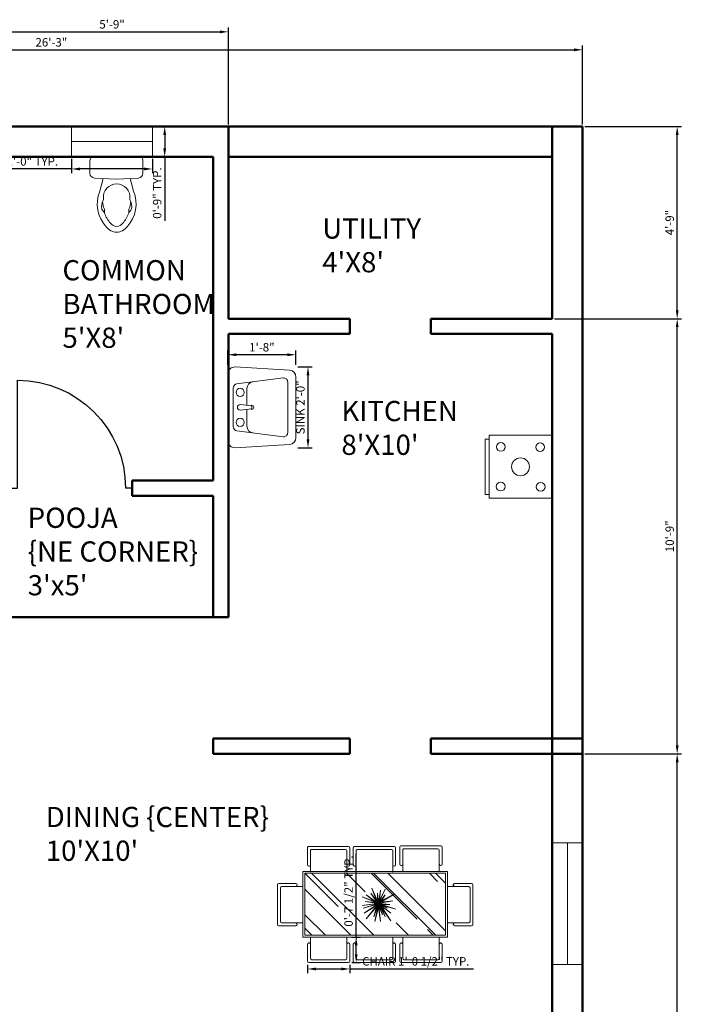
# Model space of a CAD drawing. Units: inches. Extents: x 20697 to 21575, y 6189 to 6822.
# Tile 4 of 7: x 20866 to 21063, y 6490 to 6782. Entities that reach past the tile are written whole.
import ezdxf

# ---------------------------------------------------------------- set-up
doc = ezdxf.new("R2010")
doc.units = ezdxf.units.IN
for name, color, linetype, lineweight in [('A-ANNO-DIMS', 2, 'Continuous', 18), ('A-AREA-IDEN', 7, 'Continuous', 18), ('A-DOOR', 4, 'Continuous', 25), ('A-EQPM', 9, 'Continuous', 18), ('A-FLOR-FIXT', 9, 'Continuous', 18), ('A-FURN', 8, 'Continuous', 18), ('A-GLAZ', 4, 'Continuous', 18), ('A-WALL', 7, 'Continuous', 50)]:
    doc.layers.add(name, color=color, linetype=linetype, lineweight=lineweight)
doc.styles.get("Standard").update_dxf_attribs({"font": 'arial.ttf'})
doc.dimstyles.new('ISO-25', dxfattribs={"dimtxt": 2.5, "dimasz": 2.5, "dimexe": 1.25, "dimexo": 0.625, "dimtad": 1, "dimdec": 0, "dimlunit": 3, "dimtxsty": 'Standard', "dimcen": 2.5, "dimadec": 0, "dimazin": 0, "dimtfac": 1, "dimtdec": 0, "dimtmove": 0, "dimatfit": 3, "dimfxl": 1, "dimarcsym": 0})

# ---------------------------------------------------------------- blocks, each defined once
blk = doc.blocks.new('*D5')
at = {"layer": 'A-ANNO-DIMS', "color": 0, "lineweight": -2, "transparency": 16777216}
for p, q in [((20718.29, 6750.68), (20718.29, 6774.03)), ((20720.79, 6772.78), (21030.79, 6772.78)), ((21033.29, 6750.68), (21033.29, 6774.03))]:
    blk.add_line(p, q, dxfattribs=at)
at = {"layer": 'A-ANNO-DIMS', "color": 0, "transparency": 16777216}
for points in [[(20720.79, 6773.19), (20720.79, 6772.36), (20718.29, 6772.78)], [(21030.79, 6773.19), (21030.79, 6772.36), (21033.29, 6772.78)]]:
    blk.add_solid(points, dxfattribs=at)
at = {"layer": 'Defpoints', "color": 0, "transparency": 16777216}
for p in [(21033.29, 6772.78), (20718.29, 6750.06), (21033.29, 6750.06)]:
    blk.add_point(p, dxfattribs=at)
at = {"layer": 'A-ANNO-DIMS', "color": 0, "transparency": 16777216, "insert": (20875.79, 6774.68), "char_height": 2.5, "attachment_point": 5}
blk.add_mtext('26\'-3"', dxfattribs=at)
blk = doc.blocks.new('A$C1308471B')
at = {"ltscale": 20}
for p, q in [((0, 0.4607), (0, 0.0186)), ((0.0354, 0.4793), (0.1495, 0.4793)), ((0.2013, 0.2397), (0.1923, 0.4384)), ((0.1957, 0.3639), (0.3109, 0.3953)), ((0.4982, 0.3575), (0.4822, 0.3709)), ((0.5021, 0.3528), (0.4724, 0.3528)), ((0.2013, 0.2397), (0.1923, 0.0409)), ((0.1959, 0.1193), (0.3109, 0.0879)), ((0.5021, 0.1304), (0.4724, 0.1304)), ((0.4982, 0.1257), (0.4822, 0.1123)), ((0.0354, 0), (0.1495, 0))]:
    blk.add_line(p, q, dxfattribs=at)
for centre, radius, start, end in [((0.006, 0.4607), 0.006, 136.52689, 180), ((0.0354, 0.4328), 0.0465, 90, 136.52689), ((0.1495, 0.4365), 0.0429, 2.57554, 90), ((0.3654, 0.2416), 0.1206, 83.35226, 180), ((0.4248, 0.1104), 0.3068, 47.41345, 111.79241), ((0.3823, 0.3868), 0.0255, 263.35226, 298.57415), ((0.4494, 0.2636), 0.1148, 79.39683, 118.57415), ((0.405, 0.2159), 0.153, 63.50202, 90.45216), ((0.4658, 0.3513), 0.0255, 50, 79.39683), ((0.5146, 0.377), 0.0255, 230, 251.38812), ((0.5021, 0.3273), 0.0255, 70.3751, 90), ((0.4248, 0.1104), 0.2558, 46.61198, 70.3751), ((0.5654, 0.2416), 0.065, 0, 57.29738), ((0.5654, 0.2416), 0.116, 0, 54.71147), ((0.3654, 0.2416), 0.1206, 180, 276.64774), ((0.4248, 0.3728), 0.2558, 289.6249, 313.38802), ((0.5654, 0.2416), 0.065, 302.70262, 0), ((0.5654, 0.2416), 0.116, 305.28853, 0), ((0.4248, 0.3728), 0.3068, 248.20759, 312.58655), ((0.3823, 0.0964), 0.0255, 61.42585, 96.64774), ((0.4494, 0.2196), 0.1148, 241.42585, 280.60317), ((0.405, 0.2673), 0.153, 269.54784, 296.49798), ((0.4658, 0.1319), 0.0255, 280.60317, 310), ((0.5146, 0.1062), 0.0255, 108.61188, 130), ((0.5021, 0.1559), 0.0255, 270, 289.6249), ((0.006, 0.0186), 0.006, 180, 223.47311), ((0.0354, 0.0465), 0.0465, 223.47311, 270), ((0.1495, 0.0429), 0.0429, 270, 357.42446)]:
    blk.add_arc(centre, radius, start, end, dxfattribs=at)
blk = doc.blocks.new('A$C2BB73538')
for p, q in [((0, 0.3474), (0.0187, 0.0365)), ((0.0388, 0.3886), (0.4225, 0.3886)), ((0.1191, 0.3575), (0.3422, 0.3575)), ((0.4613, 0.3474), (0.4427, 0.0365)), ((0.096, 0.3371), (0.063, 0.0728)), ((0.2151, 0.3186), (0.2229, 0.2526)), ((0.2384, 0.2526), (0.2462, 0.3186)), ((0.3653, 0.3371), (0.3984, 0.0728)), ((0.1231, 0.2798), (0.2197, 0.2798)), ((0.2229, 0.2526), (0.2384, 0.2526)), ((0.2416, 0.2798), (0.3382, 0.2798)), ((0.3752, 0.0466), (0.0861, 0.0466)), ((0.4039, 0), (0.0574, 0))]:
    blk.add_line(p, q)
for centre in [(0.1452, 0.3186), (0.3161, 0.3186)]:
    blk.add_circle(centre, 0.0233)
for centre, radius, start, end in [((0.0388, 0.3497), 0.0389, 90, 183.4336), ((0.1191, 0.3342), 0.0233, 90, 172.875), ((0.3422, 0.3342), 0.0233, 7.125, 90), ((0.3422, 0.3342), 0.0233, 7.125, 90), ((0.4225, 0.3497), 0.0389, 356.5664, 90), ((0.2307, 0.3186), 0.0155, 0, 180), ((0.1231, 0.2409), 0.0389, 90, 172.875), ((0.2307, 0.2526), 0.0117, 138.1701, 41.8299), ((0.3382, 0.2409), 0.0389, 7.125, 90), ((0.0861, 0.0699), 0.0233, 172.875, 270), ((0.3752, 0.0699), 0.0233, 270, 7.125), ((0.0574, 0.0389), 0.0389, 183.4336, 270), ((0.4039, 0.0389), 0.0389, 270, 356.5664)]:
    blk.add_arc(centre, radius, start, end)
blk = doc.blocks.new('DOOR-SWING-36')
for p, q in [((34, 0), (34, 32)), ((0, 0), (2, 0)), ((36, 0), (34, 0))]:
    blk.add_line(p, q)
blk.add_arc((34, 0), 32, 90, 180)
blk = doc.blocks.new('WIN-36X9')
for p, q in [((0, 9), (36, 9)), ((0, 0), (0, 9)), ((36, 9), (36, 0)), ((0, 4.5), (36, 4.5)), ((36, 0), (0, 0))]:
    blk.add_line(p, q)
blk = doc.blocks.new('WIN-24X9')
for p, q in [((0, 9), (24, 9)), ((0, 0), (0, 9)), ((24, 9), (24, 0)), ((0, 4.5), (24, 4.5)), ((24, 0), (0, 0))]:
    blk.add_line(p, q)
blk = doc.blocks.new('CHAIR-DINING')
for p, q in [((0.87, 1.26), (0.87, 7.58)), ((11.69, 7.58), (11.69, 1.26)), ((0, 0.39), (0, 5.43)), ((0.48, 5.82), (0.39, 5.82)), ((12.17, 5.82), (12.08, 5.82)), ((12.56, 5.43), (12.56, 0.39)), ((11.3, 0.87), (1.26, 0.87)), ((12.17, 0), (0.39, 0))]:
    blk.add_line(p, q)
for centre, start, end in [((0.39, 5.43), 90, 180), ((0.48, 5.43), 0, 90), ((12.08, 5.43), 90, 180), ((12.17, 5.43), 0, 90), ((0.39, 0.39), 180, 270), ((1.26, 1.26), 180, 270), ((11.3, 1.26), 270, 0), ((12.17, 0.39), 270, 0)]:
    blk.add_arc(centre, 0.39, start, end)
blk = doc.blocks.new('*D22')
at = {"layer": 'A-ANNO-DIMS', "color": 0, "lineweight": -2, "transparency": 16777216}
for p, q in [((20951.72, 6501.55), (20951.72, 6499.04)), ((20964.28, 6501.55), (20964.28, 6499.04)), ((20954.22, 6500.29), (20961.78, 6500.29)), ((20964.28, 6500.29), (21000.9, 6500.29))]:
    blk.add_line(p, q, dxfattribs=at)
at = {"layer": 'A-ANNO-DIMS', "color": 0, "transparency": 16777216}
for points in [[(20954.22, 6500.7), (20954.22, 6499.87), (20951.72, 6500.29)], [(20961.78, 6500.7), (20961.78, 6499.87), (20964.28, 6500.29)]]:
    blk.add_solid(points, dxfattribs=at)
at = {"layer": 'Defpoints', "color": 0, "transparency": 16777216}
for p in [(20951.72, 6502.17), (20964.28, 6502.17), (20964.28, 6500.29)]:
    blk.add_point(p, dxfattribs=at)
at = {"layer": 'A-ANNO-DIMS', "color": 0, "transparency": 16777216, "insert": (20983.84, 6502.21), "char_height": 2.5, "attachment_point": 5}
blk.add_mtext('CHAIR 1\'-0 1/2" TYP.', dxfattribs=at)
blk = doc.blocks.new('*D23')
at = {"layer": 'A-ANNO-DIMS', "color": 0, "lineweight": -2, "transparency": 16777216}
for p, q in [((20966.16, 6509.75), (20966.16, 6534.56)), ((20964.9, 6509.75), (20967.41, 6509.75)), ((20966.16, 6504.67), (20966.16, 6507.25)), ((20964.9, 6502.17), (20967.41, 6502.17))]:
    blk.add_line(p, q, dxfattribs=at)
at = {"layer": 'A-ANNO-DIMS', "color": 0, "transparency": 16777216}
for points in [[(20965.74, 6507.25), (20966.58, 6507.25), (20966.16, 6509.75)], [(20965.74, 6504.67), (20966.58, 6504.67), (20966.16, 6502.17)]]:
    blk.add_solid(points, dxfattribs=at)
at = {"layer": 'Defpoints', "color": 0, "transparency": 16777216}
for p in [(20964.28, 6509.75), (20966.16, 6509.75), (20964.28, 6502.17)]:
    blk.add_point(p, dxfattribs=at)
at = {"layer": 'A-ANNO-DIMS', "color": 0, "transparency": 16777216, "insert": (20964.24, 6523.4), "char_height": 2.5, "attachment_point": 5, "rotation": 90}
blk.add_mtext('0\'-7 1/2" TYP.', dxfattribs=at)
blk = doc.blocks.new('*D28')
at = {"layer": 'A-ANNO-DIMS', "color": 0, "lineweight": -2, "transparency": 16777216}
for p, q in [((20881.79, 6740.43), (20881.79, 6736.21)), ((20905.79, 6740.43), (20905.79, 6736.21)), ((20881.79, 6737.46), (20836.34, 6737.46)), ((20903.29, 6737.46), (20884.29, 6737.46))]:
    blk.add_line(p, q, dxfattribs=at)
at = {"layer": 'A-ANNO-DIMS', "color": 0, "transparency": 16777216}
for points in [[(20884.29, 6737.87), (20884.29, 6737.04), (20881.79, 6737.46)], [(20903.29, 6737.87), (20903.29, 6737.04), (20905.79, 6737.46)]]:
    blk.add_solid(points, dxfattribs=at)
at = {"layer": 'Defpoints', "color": 0, "transparency": 16777216}
for p in [(20881.79, 6741.06), (20905.79, 6741.06), (20881.79, 6737.46)]:
    blk.add_point(p, dxfattribs=at)
at = {"layer": 'A-ANNO-DIMS', "color": 0, "transparency": 16777216, "insert": (20857.81, 6739.37), "char_height": 2.5, "attachment_point": 5}
blk.add_mtext('BATH WINDOW 2\'-0" TYP.', dxfattribs=at)
blk = doc.blocks.new('*D29')
at = {"layer": 'A-ANNO-DIMS', "color": 0, "lineweight": -2, "transparency": 16777216}
for p, q in [((20906.42, 6750.06), (20910.64, 6750.06)), ((20909.39, 6747.56), (20909.39, 6743.56)), ((20906.42, 6741.06), (20910.64, 6741.06)), ((20909.39, 6741.06), (20909.39, 6722.07))]:
    blk.add_line(p, q, dxfattribs=at)
at = {"layer": 'A-ANNO-DIMS', "color": 0, "transparency": 16777216}
for points in [[(20908.98, 6747.56), (20909.81, 6747.56), (20909.39, 6750.06)], [(20908.98, 6743.56), (20909.81, 6743.56), (20909.39, 6741.06)]]:
    blk.add_solid(points, dxfattribs=at)
at = {"layer": 'Defpoints', "color": 0, "transparency": 16777216}
for p in [(20905.79, 6750.06), (20905.79, 6741.06), (20909.39, 6741.06)]:
    blk.add_point(p, dxfattribs=at)
at = {"layer": 'A-ANNO-DIMS', "color": 0, "transparency": 16777216, "insert": (20907.49, 6730.31), "char_height": 2.5, "attachment_point": 5, "rotation": 90}
blk.add_mtext('0\'-9" TYP.', dxfattribs=at)
blk = doc.blocks.new('*D50')
at = {"layer": 'A-ANNO-DIMS', "color": 0, "lineweight": -2, "transparency": 16777216}
for p, q in [((20948.91, 6678.78), (20953.14, 6678.78)), ((20951.89, 6657.28), (20951.89, 6676.28)), ((20948.91, 6654.78), (20953.14, 6654.78))]:
    blk.add_line(p, q, dxfattribs=at)
at = {"layer": 'A-ANNO-DIMS', "color": 0, "transparency": 16777216}
for points in [[(20951.47, 6676.28), (20952.3, 6676.28), (20951.89, 6678.78)], [(20951.47, 6657.28), (20952.3, 6657.28), (20951.89, 6654.78)]]:
    blk.add_solid(points, dxfattribs=at)
at = {"layer": 'Defpoints', "color": 0, "transparency": 16777216}
for p in [(20948.29, 6678.78), (20951.89, 6678.78), (20948.29, 6654.78)]:
    blk.add_point(p, dxfattribs=at)
at = {"layer": 'A-ANNO-DIMS', "color": 0, "transparency": 16777216, "insert": (20949.97, 6666.78), "char_height": 2.5, "attachment_point": 5, "rotation": 90}
blk.add_mtext('SINK 2\'-0"', dxfattribs=at)
blk = doc.blocks.new('*D51')
at = {"layer": 'A-ANNO-DIMS', "color": 0, "lineweight": -2, "transparency": 16777216}
for p, q in [((20928.13, 6679.41), (20928.13, 6683.63)), ((20945.79, 6682.38), (20930.63, 6682.38)), ((20948.29, 6679.41), (20948.29, 6683.63))]:
    blk.add_line(p, q, dxfattribs=at)
at = {"layer": 'A-ANNO-DIMS', "color": 0, "transparency": 16777216}
for points in [[(20930.63, 6682.8), (20930.63, 6681.97), (20928.13, 6682.38)], [(20945.79, 6682.8), (20945.79, 6681.97), (20948.29, 6682.38)]]:
    blk.add_solid(points, dxfattribs=at)
at = {"layer": 'Defpoints', "color": 0, "transparency": 16777216}
for p in [(20928.13, 6682.38), (20928.13, 6678.78), (20948.29, 6678.78)]:
    blk.add_point(p, dxfattribs=at)
at = {"layer": 'A-ANNO-DIMS', "color": 0, "transparency": 16777216, "insert": (20938.21, 6684.28), "char_height": 2.5, "attachment_point": 5}
blk.add_mtext('1\'-8"', dxfattribs=at)
blk = doc.blocks.new('*D57')
at = {"layer": 'A-ANNO-DIMS', "color": 0, "lineweight": -2, "transparency": 16777216}
for p, q in [((21033.92, 6564.06), (21062.59, 6564.06)), ((21061.34, 6274.06), (21061.34, 6561.56)), ((21033.92, 6271.56), (21062.59, 6271.56))]:
    blk.add_line(p, q, dxfattribs=at)
at = {"layer": 'A-ANNO-DIMS', "color": 0, "transparency": 16777216}
for points in [[(21060.93, 6561.56), (21061.76, 6561.56), (21061.34, 6564.06)], [(21060.93, 6274.06), (21061.76, 6274.06), (21061.34, 6271.56)]]:
    blk.add_solid(points, dxfattribs=at)
at = {"layer": 'Defpoints', "color": 0, "transparency": 16777216}
for p in [(21033.29, 6564.06), (21061.34, 6564.06), (21033.29, 6271.56)]:
    blk.add_point(p, dxfattribs=at)
at = {"layer": 'A-ANNO-DIMS', "color": 0, "transparency": 16777216, "insert": (21059.42, 6417.81), "char_height": 2.5, "attachment_point": 5, "rotation": 90}
blk.add_mtext('24\'-4 1/2"', dxfattribs=at)
blk = doc.blocks.new('*D58')
at = {"layer": 'A-ANNO-DIMS', "color": 0, "lineweight": -2, "transparency": 16777216}
for p, q in [((21024.92, 6693.06), (21062.59, 6693.06)), ((21061.34, 6566.56), (21061.34, 6690.56)), ((21033.92, 6564.06), (21062.59, 6564.06))]:
    blk.add_line(p, q, dxfattribs=at)
at = {"layer": 'A-ANNO-DIMS', "color": 0, "transparency": 16777216}
for points in [[(21060.93, 6690.56), (21061.76, 6690.56), (21061.34, 6693.06)], [(21060.93, 6566.56), (21061.76, 6566.56), (21061.34, 6564.06)]]:
    blk.add_solid(points, dxfattribs=at)
at = {"layer": 'Defpoints', "color": 0, "transparency": 16777216}
for p in [(21024.29, 6693.06), (21061.34, 6693.06), (21033.29, 6564.06)]:
    blk.add_point(p, dxfattribs=at)
at = {"layer": 'A-ANNO-DIMS', "color": 0, "transparency": 16777216, "insert": (21059.44, 6628.56), "char_height": 2.5, "attachment_point": 5, "rotation": 90}
blk.add_mtext('10\'-9"', dxfattribs=at)
blk = doc.blocks.new('*D59')
at = {"layer": 'A-ANNO-DIMS', "color": 0, "lineweight": -2, "transparency": 16777216}
for p, q in [((21033.92, 6750.06), (21062.59, 6750.06)), ((21061.34, 6695.56), (21061.34, 6747.56)), ((21024.92, 6693.06), (21062.59, 6693.06))]:
    blk.add_line(p, q, dxfattribs=at)
at = {"layer": 'A-ANNO-DIMS', "color": 0, "transparency": 16777216}
for points in [[(21060.93, 6747.56), (21061.76, 6747.56), (21061.34, 6750.06)], [(21060.93, 6695.56), (21061.76, 6695.56), (21061.34, 6693.06)]]:
    blk.add_solid(points, dxfattribs=at)
at = {"layer": 'Defpoints', "color": 0, "transparency": 16777216}
for p in [(21033.29, 6750.06), (21061.34, 6750.06), (21024.29, 6693.06)]:
    blk.add_point(p, dxfattribs=at)
at = {"layer": 'A-ANNO-DIMS', "color": 0, "transparency": 16777216, "insert": (21059.44, 6721.56), "char_height": 2.5, "attachment_point": 5, "rotation": 90}
blk.add_mtext('4\'-9"', dxfattribs=at)
blk = doc.blocks.new('*D61')
at = {"layer": 'A-ANNO-DIMS', "color": 0, "lineweight": -2, "transparency": 16777216}
for p, q in [((20859.29, 6750.68), (20859.29, 6779.36)), ((20861.79, 6778.11), (20925.79, 6778.11)), ((20928.29, 6750.68), (20928.29, 6779.36))]:
    blk.add_line(p, q, dxfattribs=at)
at = {"layer": 'A-ANNO-DIMS', "color": 0, "transparency": 16777216}
for points in [[(20861.79, 6778.52), (20861.79, 6777.69), (20859.29, 6778.11)], [(20925.79, 6778.52), (20925.79, 6777.69), (20928.29, 6778.11)]]:
    blk.add_solid(points, dxfattribs=at)
at = {"layer": 'Defpoints', "color": 0, "transparency": 16777216}
for p in [(20928.29, 6778.11), (20859.29, 6750.06), (20928.29, 6750.06)]:
    blk.add_point(p, dxfattribs=at)
at = {"layer": 'A-ANNO-DIMS', "color": 0, "transparency": 16777216, "insert": (20893.79, 6780.01), "char_height": 2.5, "attachment_point": 5}
blk.add_mtext('5\'-9"', dxfattribs=at)

msp = doc.modelspace()

# ---------------------------------------------------------------- linework, layer by layer
at = {"layer": 'A-EQPM'}
for p, q in [((21005.62, 6658.5), (21005.62, 6639.82)), ((21024.29, 6658.5), (21005.62, 6658.5)), ((21024.29, 6658.5), (21024.29, 6639.82)), ((21005.62, 6657.33), (21004.45, 6657.33)), ((21004.45, 6657.33), (21004.45, 6640.99)), ((21005.62, 6640.99), (21004.45, 6640.99)), ((21024.29, 6639.82), (21005.62, 6639.82))]:
    msp.add_line(p, q, dxfattribs=at)
for centre, radius in [((21009.06, 6655.06), 1.31), ((21020.72, 6654.99), 1.31), ((21014.89, 6649.16), 2.65), ((21008.99, 6643.3), 1.31), ((21020.86, 6643.23), 1.31)]:
    msp.add_circle(centre, radius, dxfattribs=at)
at = {"layer": 'A-FURN'}
for p, q in [((20950.39, 6529.22), (20950.39, 6509.73)), ((20993.21, 6529.22), (20950.39, 6529.22)), ((20950.93, 6528.68), (20950.93, 6510.28)), ((20992.67, 6528.68), (20950.93, 6528.68)), ((20960.82, 6518.8), (20950.94, 6528.68)), ((20971.36, 6510.28), (20952.96, 6528.68)), ((20968.82, 6523.11), (20963.25, 6528.68)), ((20984.25, 6515.03), (20970.6, 6528.68)), ((20989.74, 6510.28), (20971.33, 6528.68)), ((20992.67, 6511.57), (20975.56, 6528.68)), ((20990.31, 6526.24), (20987.87, 6528.68)), ((20992.67, 6525.71), (20989.7, 6528.68)), ((20992.67, 6510.28), (20992.67, 6528.68)), ((20993.21, 6509.73), (20993.21, 6529.22)), ((20942.81, 6525.24), (20942.81, 6513.47)), ((20948.25, 6525.63), (20943.2, 6525.63)), ((20943.68, 6524.38), (20943.68, 6514.33)), ((20950.39, 6524.77), (20944.07, 6524.77)), ((20948.64, 6525.24), (20948.64, 6525.16)), ((20972.8, 6519.68), (20970.82, 6524.21)), ((20970.82, 6524.21), (20972.23, 6520.53)), ((20993.21, 6524.77), (20999.53, 6524.77)), ((20994.96, 6525.24), (20994.96, 6525.16)), ((20995.35, 6525.63), (21000.4, 6525.63)), ((20999.92, 6524.38), (20999.92, 6514.33)), ((21000.79, 6525.24), (21000.79, 6513.47)), ((20964.57, 6510.28), (20950.93, 6523.91)), ((20972.8, 6519.68), (20967.99, 6521.66)), ((20967.99, 6521.66), (20971.67, 6520.25)), ((20972.8, 6519.68), (20969.12, 6522.23)), ((20971.67, 6520.25), (20969.12, 6522.23)), ((20972.8, 6519.68), (20970.54, 6522.79)), ((20970.54, 6522.79), (20972.23, 6520.25)), ((20972.8, 6519.68), (20972.52, 6522.79)), ((20972.52, 6522.79), (20972.52, 6520.53)), ((20972.8, 6519.68), (20974.78, 6523.92)), ((20972.8, 6519.68), (20973.37, 6523.64)), ((20972.8, 6519.68), (20977.61, 6522.51)), ((20972.8, 6519.68), (20974.78, 6522.23)), ((20973.08, 6520.53), (20974.78, 6523.92)), ((20973.37, 6523.64), (20973.08, 6520.53)), ((20974.78, 6522.23), (20973.41, 6520.04)), ((20977.61, 6522.51), (20973.75, 6520.58)), ((20974.78, 6523.92), (20974.78, 6523.92)), ((20967.99, 6519.11), (20972.23, 6519.68)), ((20972.8, 6519.68), (20967.99, 6519.11)), ((20972.8, 6519.68), (20968.27, 6518.27)), ((20968.27, 6518.27), (20972.23, 6519.4)), ((20972.8, 6519.68), (20968.56, 6516.85)), ((20968.56, 6516.85), (20972.23, 6519.11)), ((20968.84, 6520.25), (20971.95, 6519.96)), ((20972.8, 6519.68), (20968.84, 6520.25)), ((20972.8, 6519.68), (20969.12, 6515.15)), ((20969.12, 6515.15), (20972.17, 6518.68)), ((20972.8, 6519.68), (20971.38, 6515.72)), ((20971.38, 6515.72), (20972.17, 6518.68)), ((20972.8, 6519.68), (20971.67, 6514.31)), ((20972.8, 6518.55), (20971.67, 6514.31)), ((20972.8, 6519.68), (20977.04, 6520.53)), ((20972.8, 6519.68), (20973.37, 6514.31)), ((20972.8, 6519.68), (20976.19, 6519.4)), ((20972.8, 6519.68), (20974.78, 6515.72)), ((20972.8, 6519.68), (20973.93, 6516.29)), ((20972.8, 6519.68), (20976.48, 6516.85)), ((20972.8, 6519.68), (20975.35, 6518.27)), ((20972.8, 6519.68), (20976.48, 6514.59)), ((20972.8, 6519.68), (20977.89, 6517.98)), ((20973.37, 6514.31), (20972.8, 6518.55)), ((20973.93, 6516.29), (20972.88, 6518.91)), ((20976.48, 6516.85), (20973.08, 6519.4)), ((20977.04, 6520.53), (20973.41, 6520.04)), ((20976.19, 6519.4), (20973.65, 6519.4)), ((20976.48, 6514.59), (20973.65, 6518.83)), ((20974.78, 6515.72), (20973.69, 6518.45)), ((20975.35, 6518.27), (20974.21, 6519.11)), ((20977.89, 6517.98), (20974.21, 6519.11)), ((20957.03, 6510.28), (20950.93, 6516.38)), ((20943.2, 6513.08), (20948.25, 6513.08)), ((20944.07, 6513.94), (20950.39, 6513.94)), ((20948.64, 6513.55), (20948.64, 6513.47)), ((20981.65, 6510.28), (20978, 6513.93)), ((20999.53, 6513.94), (20993.21, 6513.94)), ((20994.96, 6513.55), (20994.96, 6513.47)), ((21000.4, 6513.08), (20995.35, 6513.08)), ((20950.39, 6509.73), (20993.21, 6509.73)), ((20952.99, 6510.28), (20950.93, 6512.34)), ((20950.93, 6510.28), (20992.67, 6510.28)), ((20989, 6510.28), (20987.28, 6512))]:
    msp.add_line(p, q, dxfattribs=at)
for centre, start, end in [((20943.2, 6525.24), 90, 180), ((20944.07, 6524.38), 90, 180), ((20948.25, 6525.24), 0, 90), ((20948.25, 6525.16), 270, 0), ((20995.35, 6525.24), 90, 180), ((20995.35, 6525.16), 180, 270), ((20999.53, 6524.38), 0, 90), ((21000.4, 6525.24), 0, 90), ((20943.2, 6513.47), 180, 270), ((20944.07, 6514.33), 180, 270), ((20948.25, 6513.47), 270, 90.0583), ((20995.35, 6513.55), 90, 269.8631), ((20999.53, 6514.33), 270, 0), ((21000.4, 6513.47), 270, 0)]:
    msp.add_arc(centre, 0.39, start, end, dxfattribs=at)
at = {"layer": 'A-WALL'}
for p, q in [((20718.29, 6750.06), (21033.29, 6750.06)), ((20928.29, 6750.06), (20928.29, 6693.06)), ((21024.29, 6750.06), (21024.29, 6693.06)), ((21033.29, 6750.06), (21033.29, 6238.56)), ((20863.79, 6741.06), (20923.79, 6741.06)), ((20923.79, 6741.06), (20923.79, 6645.06)), ((20928.29, 6741.06), (21024.29, 6741.06)), ((20928.29, 6693.06), (20964.29, 6693.06)), ((20964.29, 6688.56), (20964.29, 6693.06)), ((20988.29, 6688.56), (20988.29, 6693.06)), ((20988.29, 6693.06), (21024.29, 6693.06)), ((20928.29, 6688.56), (20964.29, 6688.56)), ((20928.29, 6688.56), (20928.29, 6604.56)), ((20988.29, 6688.56), (21024.29, 6688.56)), ((21024.29, 6688.56), (21024.29, 6280.56)), ((20899.79, 6645.06), (20923.79, 6645.06)), ((20899.79, 6645.06), (20899.79, 6640.56)), ((20899.79, 6640.56), (20923.79, 6640.56)), ((20923.79, 6640.56), (20923.79, 6604.56)), ((20863.79, 6604.56), (20928.29, 6604.56)), ((20923.79, 6568.56), (20964.29, 6568.56)), ((20923.79, 6568.56), (20923.79, 6564.06)), ((20964.29, 6568.56), (20964.29, 6564.06)), ((20988.29, 6568.56), (21033.29, 6568.56)), ((20988.29, 6568.56), (20988.29, 6564.06)), ((20923.79, 6564.06), (20964.29, 6564.06)), ((20988.29, 6564.06), (21033.29, 6564.06))]:
    msp.add_line(p, q, dxfattribs=at)

# ---------------------------------------------------------------- block references
at = {"layer": 'A-DOOR', "extrusion": (0, 0, -1), "zscale": -1}
msp.add_blockref('DOOR-SWING-36', (-20899.79, 6642.81), dxfattribs=at)
at = {"layer": 'A-FLOR-FIXT'}
for name, p, xscale, yscale, zscale, rotation in [('A$C1308471B', (20887.24, 6741.06), 32.76079773388695, 32.76079773388695, 32.76079773388695, 269.9999999999999), ('A$C2BB73538', (20948.29, 6654.82), 51.87621955604623, 51.87621955604623, 51.87621955604623, 90)]:
    msp.add_blockref(name, p, dxfattribs=dict(at, xscale=xscale, yscale=yscale, zscale=zscale, rotation=rotation))
at = {"layer": 'A-FURN', "rotation": 180}
for p in [(20964.28, 6536.61), (20977.87, 6536.61), (20991.68, 6536.78)]:
    msp.add_blockref('CHAIR-DINING', p, dxfattribs=at)
at = {"layer": 'A-FURN'}
for p in [(20951.72, 6502.17), (20965.31, 6502.17), (20979.12, 6502.17)]:
    msp.add_blockref('CHAIR-DINING', p, dxfattribs=at)
at = {"layer": 'A-GLAZ'}
for name, p, rotation in [('WIN-24X9', (20905.79, 6750.06), 180), ('WIN-36X9', (21024.29, 6537.64), 270.0000000000129)]:
    msp.add_blockref(name, p, dxfattribs=dict(at, rotation=rotation))

# ---------------------------------------------------------------- texts
at = {"layer": 'A-AREA-IDEN', "char_height": 6, "attachment_point": 1}
for s, insert in [("UTILITY\\P4'X8'", (20956.11, 6722.81)), ("COMMON \\PBATHROOM\\P5'X8'", (20879.08, 6710.43)), ("KITCHEN\\P8'X10'", (20961.79, 6668.69)), ("DINING \\{CENTER\\}\\P10'X10'", (20874.14, 6548.34))]:
    msp.add_mtext(s, dxfattribs=dict(at, insert=insert))
at = {"layer": 'A-AREA-IDEN', "insert": (20868.78, 6637.05), "char_height": 6, "width": 109.5282, "attachment_point": 1}
msp.add_mtext("POOJA\\P\\{NE CORNER\\}\\P3'x5'", dxfattribs=at)

# ---------------------------------------------------------------- dimensions: what is measured, and where the dimension line sits
at = {"layer": 'A-ANNO-DIMS'}
for base, p1, p2, override, picture, middle in [((20928.29, 6778.11), (20859.29, 6750.06), (20928.29, 6750.06), {"dimdec": 1, "dimlfac": 1, "dimrnd": 0, "dimzin": 1, "dimdsep": 46, "dimlunit": 4, "dimfrac": 2}, '*D61', (20893.79, 6780.01)), ((21033.29, 6772.78), (20718.29, 6750.06), (21033.29, 6750.06), {"dimclrd": 0, "dimclre": 0, "dimclrt": 0}, '*D5', (20875.79, 6774.68))]:
    dim = msp.add_linear_dim(base=base, p1=p1, p2=p2, dimstyle='ISO-25', override=override, dxfattribs=at)
    dim.commit()
    dim.dimension.update_dxf_attribs({"geometry": picture, "text_midpoint": middle})
for base, p1, p2, angle, text, picture, middle in [((20909.39, 6741.06), (20905.79, 6750.06), (20905.79, 6741.06), 270, '<> TYP.', '*D29', (20907.49, 6730.31)), ((20881.79, 6737.46), (20905.79, 6741.06), (20881.79, 6741.06), 180, 'BATH WINDOW <> TYP.', '*D28', (20857.81, 6739.37)), ((20951.89, 6678.78), (20948.29, 6654.78), (20948.29, 6678.78), 90, 'SINK <>', '*D50', (20949.97, 6666.78)), ((20966.16, 6509.75), (20964.28, 6502.17), (20964.28, 6509.75), 90, '<> TYP.', '*D23', (20964.24, 6523.4))]:
    dim = msp.add_linear_dim(base=base, p1=p1, p2=p2, angle=angle, text=text, dimstyle='ISO-25', override={"dimdec": 1, "dimlfac": 1, "dimrnd": 0, "dimzin": 1, "dimdsep": 46, "dimlunit": 4, "dimfrac": 2}, dxfattribs=at)
    dim.commit()
    dim.dimension.update_dxf_attribs({"geometry": picture, "text_midpoint": middle})
for base, p1, p2, angle, picture, middle in [((21061.34, 6750.06), (21024.29, 6693.06), (21033.29, 6750.06), 90, '*D59', (21059.44, 6721.56)), ((21061.34, 6693.06), (21033.29, 6564.06), (21024.29, 6693.06), 90, '*D58', (21059.44, 6628.56)), ((20928.13, 6682.38), (20948.29, 6678.78), (20928.13, 6678.78), 180, '*D51', (20938.21, 6684.28)), ((21061.34, 6564.06), (21033.29, 6271.56), (21033.29, 6564.06), 90, '*D57', (21059.42, 6417.81))]:
    dim = msp.add_linear_dim(base=base, p1=p1, p2=p2, angle=angle, dimstyle='ISO-25', override={"dimdec": 1, "dimlfac": 1, "dimrnd": 0, "dimzin": 1, "dimdsep": 46, "dimlunit": 4, "dimfrac": 2}, dxfattribs=at)
    dim.commit()
    dim.dimension.update_dxf_attribs({"geometry": picture, "text_midpoint": middle})
dim = msp.add_linear_dim(base=(20964.28, 6500.29), p1=(20951.72, 6502.17), p2=(20964.28, 6502.17), text='CHAIR <> TYP.', dimstyle='ISO-25', override={"dimdec": 1, "dimlfac": 1, "dimrnd": 0, "dimzin": 1, "dimdsep": 46, "dimlunit": 4, "dimfrac": 2}, dxfattribs=at)
dim.commit()
dim.dimension.update_dxf_attribs({"geometry": '*D22', "text_midpoint": (20983.84, 6502.21)})

doc.saveas('drawing.dxf')
